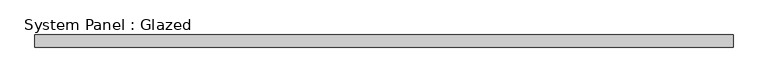
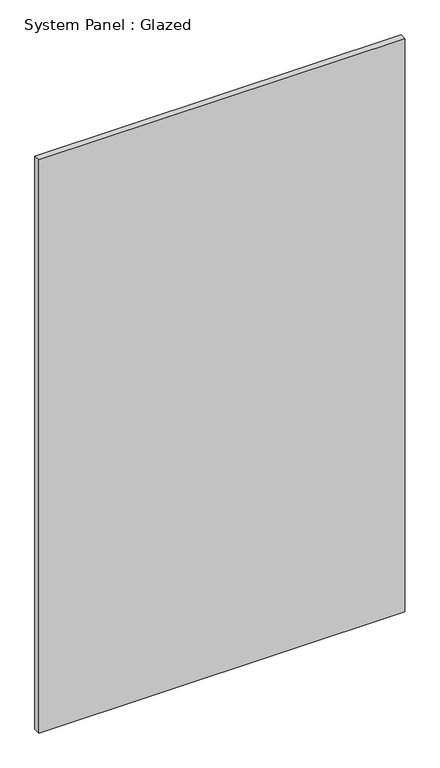
"""IFC4 building model written with IfcOpenShell, lengths in millimetres: plate geometry, System Panel : Glazed."""

from ifc_helpers import new_model, si_unit, origin, origin_with_axes, place, context, project, spatial, polyline, outline, extrude, source, transform, mapped, element, save


def system_panel_glazed_fd42546f(model_context):
    return source(origin(), model_context, "Body", "SweptSolid", [
        extrude(outline(polyline([(708.025, 19.05), (-708.025, 19.05), (-708.025, 44.45), (708.025, 44.45), (708.025, 19.05)])), origin_with_axes(), (0.0, 0.0, 1.0), 2343.15),
    ])


if __name__ == "__main__":
    model = new_model("IFC4")
    model_context = context("Model", 3, world=origin())
    ifc_project = project(units=[si_unit("LENGTHUNIT", "METRE", prefix="MILLI")], contexts=[model_context])
    site = spatial("IfcSite", under=ifc_project)
    building = spatial("IfcBuilding", under=site)
    placement = place(None, origin())
    system_panel_glazed_shape = system_panel_glazed_fd42546f(model_context)
    element("IfcPlate", 1, ObjectType="System Panel : Glazed", at=placement, inside=building, context=model_context, shape_type="MappedRepresentation", body=[
        mapped(system_panel_glazed_shape, transform((0.0, 0.0, 0.0), x_axis=(1.0, 0.0, 0.0), y_axis=(0.0, 1.0, 0.0), z_axis=(0.0, 0.0, 1.0))),
    ])
    save(model, "model.ifc")

# Revit data of these elements
# Type "System Panel : Glazed"
#   Construction Type Id = "GSP4R"
#   Analytic Construction = "1/8 in Pilkington single glazing"
#   Visual Light Transmittance = 0.9
#   Solar Heat Gain Coefficient = 0.86
#   Heat Transfer Coefficient (U) = 1.18115 BTU/(h·ft²·°F)
# Element 1 (IfcPlate, "System Panel : Glazed")
#   Materials on its faces: "Glass"
# Materials
#   "Glass": class "Glass", colour RGB 0 128 192, transparency 0.75, Description = "Soda Lime Glass", Cost = 0
